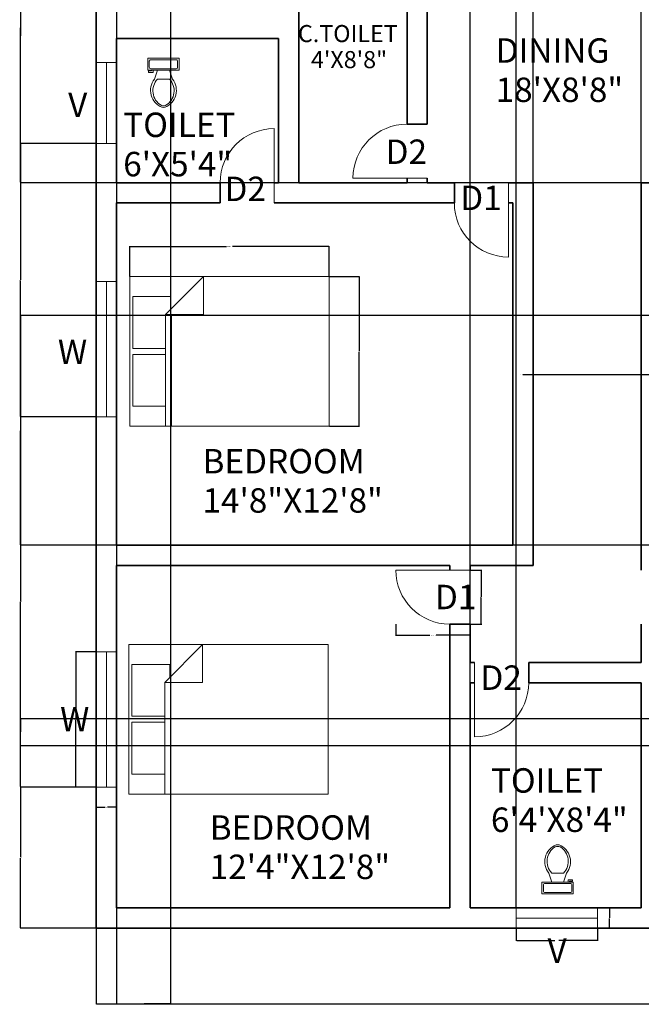
# Model space of a CAD drawing. Units: feet. Extents: x 1681 to 2398, y 1737 to 2411.
# Tile 1 of 4: x 1681 to 1957, y 1737 to 2174. Entities that reach past the tile are written whole.
import ezdxf

# ---------------------------------------------------------------- set-up
doc = ezdxf.new("R2010")
doc.units = ezdxf.units.FT
for name, color, linetype, lineweight in [('A-ANNO-DIMS', 2, 'Continuous', 18), ('A-ANNO-TEXT', 7, 'Continuous', 18), ('A-AREA-IDEN', 7, 'Continuous', 18), ('A-DOOR', 3, 'Continuous', 18), ('A-FLOR-FIXT', 9, 'Continuous', 18), ('A-FURN', 8, 'Continuous', 13), ('A-GLAZ', 4, 'Continuous', 18), ('A-WALL', 7, 'Continuous', 35)]:
    doc.layers.add(name, color=color, linetype=linetype, lineweight=lineweight)
doc.styles.get("Standard").update_dxf_attribs({"font": 'arial.ttf'})
doc.dimstyles.get("Standard").update_dxf_attribs({"dimtxt": 0.18, "dimasz": 0.18, "dimexe": 0.18, "dimexo": 0.0625, "dimgap": 0.09, "dimtad": 0, "dimtih": 1, "dimtoh": 1, "dimdec": 4, "dimzin": 0, "dimdsep": 46, "dimtxsty": 'Standard', "dimcen": 0.09, "dimadec": 0, "dimazin": 0, "dimtfac": 1, "dimtdec": 4, "dimtofl": 0, "dimtmove": 0, "dimatfit": 3, "dimfxl": 1, "dimtolj": 1, "dimtzin": 0, "dimarcsym": 0})

# ---------------------------------------------------------------- blocks, each defined once
blk = doc.blocks.new('Toilet - top')
for p, q in [((9.5, -6), (9.5, -2)), ((-10, -8.5), (-8, -8.5)), ((-10, -9.5), (-10, -8.5)), ((-7, -9.5), (-10, -9.5)), ((-8, -8.5), (-8, -8)), ((-7, -8), (-7, -9.5)), ((-4, -8), (-6, -14)), ((4, -8), (6, -14)), ((4, -14), (-4, -14))]:
    blk.add_line(p, q)
blk.add_lwpolyline([(10.5, -8), (10.5, 0), (-10.5, 0), (-10.5, -8)], close=True)
for points in [[(-9.5, -2), (-9.5, -6)], [(8.5, -1), (-8.5, -1)], [(-8.5, -7), (8.5, -7)]]:
    blk.add_lwpolyline(points)
for centre, radius, start, end in [((-8.62, -1.88), 0.884, 81.8699, 188.1301), ((-8.62, -6.12), 0.884, 171.8699, 278.1301), ((8.62, -1.88), 0.884, 351.8699, 98.1301), ((8.62, -6.12), 0.884, 261.8699, 8.1301), ((3.52, -21.58), 12.17, 141.46911, 247.97143), ((4.2, -21.82), 11.33, 136.36773, 238.94682), ((-3.52, -21.58), 12.17, 292.02843, 38.53071), ((-4.2, -21.82), 11.33, 301.05301, 43.63209), ((0, -27.88), 4, 245.73182, 294.26817), ((0, -29), 4, 254.86053, 285.13947)]:
    blk.add_arc(centre, radius, start, end)
blk = doc.blocks.new('Bed - Queen')
for p, q in [((0, -80.00003), (0, 0)), ((0, 0), (59.99999, 0)), ((59.99999, 0), (59.99999, -80.00003)), ((7.99999, -1.2), (28.79998, -1.2)), ((7.99999, -14.4), (7.99999, -1.2)), ((28.79998, -1.2), (28.79998, -14.4)), ((31.19999, -1.2), (51.99999, -1.2)), ((31.19999, -14.4), (31.19999, -1.2)), ((51.99999, -1.2), (51.99999, -16.4)), ((0, -14.4), (44.8, -14.4)), ((59.99999, -29.6), (44.8, -14.4)), ((44.8, -14.4), (44.8, -29.6)), ((44.8, -16.8), (0, -16.8)), ((51.99999, -16.4), (46.79936, -16.4)), ((44.8, -29.6), (59.99999, -29.6)), ((59.99999, -80.00003), (0, -80.00003))]:
    blk.add_line(p, q)
blk = doc.blocks.new('DOOR-SINGLE-SWING')
blk.add_line((33, 0), (0, 0))
blk.add_arc((9, 0), 24, 0, 90)
blk = doc.blocks.new('WINDOW-STANDARD')
for p, q in [((0, 9), (0, 0)), ((60, 9), (60, 0)), ((0, 4.5), (60, 4.5))]:
    blk.add_line(p, q)
blk = doc.blocks.new('WINDOW-VENTILATOR')
for p, q in [((0, 9), (0, 0)), ((36, 9), (36, 0)), ((0, 4.5), (36, 4.5))]:
    blk.add_line(p, q)
blk = doc.blocks.new('*D14')
at = {"layer": 'A-ANNO-DIMS', "color": 0, "lineweight": -2, "transparency": 16777216}
for p, q in [((1847.74, 1905.99), (1847.74, 1900.92)), ((1880.74, 1905.99), (1880.74, 1900.92)), ((1847.92, 1901.1), (1862.8, 1901.1)), ((1880.56, 1901.1), (1865.68, 1901.1))]:
    blk.add_line(p, q, dxfattribs=at)
at = {"layer": 'A-ANNO-DIMS', "color": 0, "transparency": 16777216}
for points in [[(1847.92, 1901.13), (1847.92, 1901.07), (1847.74, 1901.1)], [(1880.56, 1901.13), (1880.56, 1901.07), (1880.74, 1901.1)]]:
    blk.add_solid(points, dxfattribs=at)
at = {"layer": 'Defpoints', "color": 0, "transparency": 16777216}
for p in [(1847.74, 1906.05), (1880.74, 1906.05), (1847.74, 1901.1)]:
    blk.add_point(p, dxfattribs=at)
at = {"layer": 'A-ANNO-DIMS', "color": 0, "transparency": 16777216, "insert": (1864.24, 1901.1), "char_height": 0.18, "attachment_point": 5}
blk.add_mtext('\\A1;SINGLE DOOR 33 TYP.', dxfattribs=at)
blk = doc.blocks.new('*D15')
at = {"layer": 'A-ANNO-DIMS', "color": 0, "lineweight": -2, "transparency": 16777216}
for p, q in [((1880.8, 1930.05), (1885.87, 1930.05)), ((1885.69, 1929.87), (1885.69, 1918.23)), ((1885.69, 1906.23), (1885.69, 1917.87)), ((1880.8, 1906.05), (1885.87, 1906.05))]:
    blk.add_line(p, q, dxfattribs=at)
at = {"layer": 'A-ANNO-DIMS', "color": 0, "transparency": 16777216}
for points in [[(1885.66, 1929.87), (1885.72, 1929.87), (1885.69, 1930.05)], [(1885.66, 1906.23), (1885.72, 1906.23), (1885.69, 1906.05)]]:
    blk.add_solid(points, dxfattribs=at)
at = {"layer": 'Defpoints', "color": 0, "transparency": 16777216}
for p in [(1880.74, 1930.05), (1880.74, 1906.05), (1885.69, 1906.05)]:
    blk.add_point(p, dxfattribs=at)
at = {"layer": 'A-ANNO-DIMS', "color": 0, "transparency": 16777216, "insert": (1885.69, 1918.05), "char_height": 0.18, "attachment_point": 5}
blk.add_mtext('\\A1;24 TYP.', dxfattribs=at)
blk = doc.blocks.new('*D16')
at = {"layer": 'A-ANNO-DIMS', "color": 0, "lineweight": -2, "transparency": 16777216}
for p, q in [((1714.68, 1893.73), (1705.56, 1893.73)), ((1705.74, 1893.55), (1705.74, 1863.91)), ((1705.74, 1833.91), (1705.74, 1863.54)), ((1714.68, 1833.73), (1705.56, 1833.73))]:
    blk.add_line(p, q, dxfattribs=at)
at = {"layer": 'A-ANNO-DIMS', "color": 0, "transparency": 16777216}
for points in [[(1705.71, 1893.55), (1705.77, 1893.55), (1705.74, 1893.73)], [(1705.71, 1833.91), (1705.77, 1833.91), (1705.74, 1833.73)]]:
    blk.add_solid(points, dxfattribs=at)
at = {"layer": 'Defpoints', "color": 0, "transparency": 16777216}
for p in [(1714.74, 1893.73), (1705.74, 1833.73), (1714.74, 1833.73)]:
    blk.add_point(p, dxfattribs=at)
at = {"layer": 'A-ANNO-DIMS', "color": 0, "transparency": 16777216, "insert": (1705.74, 1863.73), "char_height": 0.18, "attachment_point": 5}
blk.add_mtext('\\A1;WINDOW 60 TYP.', dxfattribs=at)
blk = doc.blocks.new('*D17')
at = {"layer": 'A-ANNO-DIMS', "color": 0, "lineweight": -2, "transparency": 16777216}
for p, q in [((1714.74, 1833.67), (1714.74, 1824.55)), ((1723.74, 1833.67), (1723.74, 1824.55)), ((1714.92, 1824.73), (1718.78, 1824.73)), ((1723.56, 1824.73), (1719.7, 1824.73))]:
    blk.add_line(p, q, dxfattribs=at)
at = {"layer": 'A-ANNO-DIMS', "color": 0, "transparency": 16777216}
for points in [[(1714.92, 1824.76), (1714.92, 1824.7), (1714.74, 1824.73)], [(1723.56, 1824.76), (1723.56, 1824.7), (1723.74, 1824.73)]]:
    blk.add_solid(points, dxfattribs=at)
at = {"layer": 'Defpoints', "color": 0, "transparency": 16777216}
for p in [(1714.74, 1833.73), (1723.74, 1833.73), (1723.74, 1824.73)]:
    blk.add_point(p, dxfattribs=at)
at = {"layer": 'A-ANNO-DIMS', "color": 0, "transparency": 16777216, "insert": (1719.24, 1824.73), "char_height": 0.18, "attachment_point": 5}
blk.add_mtext('\\A1;9 TYP.', dxfattribs=at)
blk = doc.blocks.new('*D18')
at = {"layer": 'A-ANNO-DIMS', "color": 0, "lineweight": -2, "transparency": 16777216}
for p, q in [((1729.63, 2060.43), (1729.63, 2073.83)), ((1729.81, 2073.65), (1772.6, 2073.65)), ((1818, 2073.65), (1775.21, 2073.65)), ((1818.18, 2060.43), (1818.18, 2073.83))]:
    blk.add_line(p, q, dxfattribs=at)
at = {"layer": 'A-ANNO-DIMS', "color": 0, "transparency": 16777216}
for points in [[(1729.81, 2073.68), (1729.81, 2073.62), (1729.63, 2073.65)], [(1818, 2073.68), (1818, 2073.62), (1818.18, 2073.65)]]:
    blk.add_solid(points, dxfattribs=at)
at = {"layer": 'Defpoints', "color": 0, "transparency": 16777216}
for p in [(1729.63, 2073.65), (1729.63, 2060.36), (1818.18, 2060.36)]:
    blk.add_point(p, dxfattribs=at)
at = {"layer": 'A-ANNO-DIMS', "color": 0, "transparency": 16777216, "insert": (1773.9, 2073.65), "char_height": 0.18, "attachment_point": 5}
blk.add_mtext('\\A1;QUEEN BED 89 TYP.', dxfattribs=at)
blk = doc.blocks.new('*D19')
at = {"layer": 'A-ANNO-DIMS', "color": 0, "lineweight": -2, "transparency": 16777216}
for p, q in [((1818.24, 2060.36), (1831.64, 2060.36)), ((1831.46, 2060.18), (1831.46, 2027.34)), ((1831.46, 1994.14), (1831.46, 2026.98)), ((1818.24, 1993.96), (1831.64, 1993.96))]:
    blk.add_line(p, q, dxfattribs=at)
at = {"layer": 'A-ANNO-DIMS', "color": 0, "transparency": 16777216}
for points in [[(1831.43, 2060.18), (1831.49, 2060.18), (1831.46, 2060.36)], [(1831.43, 1994.14), (1831.49, 1994.14), (1831.46, 1993.96)]]:
    blk.add_solid(points, dxfattribs=at)
at = {"layer": 'Defpoints', "color": 0, "transparency": 16777216}
for p in [(1818.18, 2060.36), (1831.46, 2060.36), (1818.18, 1993.96)]:
    blk.add_point(p, dxfattribs=at)
at = {"layer": 'A-ANNO-DIMS', "color": 0, "transparency": 16777216, "insert": (1831.46, 2027.16), "char_height": 0.18, "attachment_point": 5}
blk.add_mtext('\\A1;66 TYP.', dxfattribs=at)
blk = doc.blocks.new('*D22')
at = {"layer": 'A-ANNO-DIMS', "color": 0, "lineweight": -2, "transparency": 16777216}
for p, q in [((1901.24, 1770.99), (1901.24, 1765.47)), ((1937.24, 1770.99), (1937.24, 1765.47)), ((1901.42, 1765.65), (1918.34, 1765.65)), ((1937.06, 1765.65), (1920.14, 1765.65))]:
    blk.add_line(p, q, dxfattribs=at)
at = {"layer": 'A-ANNO-DIMS', "color": 0, "transparency": 16777216}
for points in [[(1901.42, 1765.68), (1901.42, 1765.62), (1901.24, 1765.65)], [(1937.06, 1765.68), (1937.06, 1765.62), (1937.24, 1765.65)]]:
    blk.add_solid(points, dxfattribs=at)
at = {"layer": 'Defpoints', "color": 0, "transparency": 16777216}
for p in [(1901.24, 1771.05), (1937.24, 1771.05), (1937.24, 1765.65)]:
    blk.add_point(p, dxfattribs=at)
at = {"layer": 'A-ANNO-DIMS', "color": 0, "transparency": 16777216, "insert": (1919.24, 1765.65), "char_height": 0.18, "attachment_point": 5}
blk.add_mtext('\\A1;VENT 36 TYP.', dxfattribs=at)
blk = doc.blocks.new('*D23')
at = {"layer": 'A-ANNO-DIMS', "color": 0, "lineweight": -2, "transparency": 16777216}
for p, q in [((1937.3, 1780.05), (1942.82, 1780.05)), ((1942.64, 1779.87), (1942.64, 1775.73)), ((1942.64, 1771.23), (1942.64, 1775.37)), ((1937.3, 1771.05), (1942.82, 1771.05))]:
    blk.add_line(p, q, dxfattribs=at)
at = {"layer": 'A-ANNO-DIMS', "color": 0, "transparency": 16777216}
for points in [[(1942.61, 1779.87), (1942.67, 1779.87), (1942.64, 1780.05)], [(1942.61, 1771.23), (1942.67, 1771.23), (1942.64, 1771.05)]]:
    blk.add_solid(points, dxfattribs=at)
at = {"layer": 'Defpoints', "color": 0, "transparency": 16777216}
for p in [(1937.24, 1780.05), (1942.64, 1780.05), (1937.24, 1771.05)]:
    blk.add_point(p, dxfattribs=at)
at = {"layer": 'A-ANNO-DIMS', "color": 0, "transparency": 16777216, "insert": (1942.64, 1775.55), "char_height": 0.18, "attachment_point": 5}
blk.add_mtext('\\A1;9 TYP.', dxfattribs=at)
blk = doc.blocks.new('*D40')
at = {"layer": 'A-ANNO-DIMS', "color": 0, "lineweight": -2, "transparency": 16777216}
for p, q in [((1714.74, 1770.99), (1714.74, 1737.27)), ((2339.74, 1770.99), (2339.74, 1737.27)), ((1714.92, 1737.45), (2026.95, 1737.45)), ((2339.56, 1737.45), (2027.53, 1737.45))]:
    blk.add_line(p, q, dxfattribs=at)
at = {"layer": 'A-ANNO-DIMS', "color": 0, "transparency": 16777216}
for points in [[(1714.92, 1737.48), (1714.92, 1737.42), (1714.74, 1737.45)], [(2339.56, 1737.48), (2339.56, 1737.42), (2339.74, 1737.45)]]:
    blk.add_solid(points, dxfattribs=at)
at = {"layer": 'Defpoints', "color": 0, "transparency": 16777216}
for p in [(1714.74, 1771.05), (2339.74, 1771.05), (2339.74, 1737.45)]:
    blk.add_point(p, dxfattribs=at)
at = {"layer": 'A-ANNO-DIMS', "color": 0, "transparency": 16777216, "insert": (2027.24, 1737.45), "char_height": 0.18, "attachment_point": 5}
blk.add_mtext('\\A1;625', dxfattribs=at)
blk = doc.blocks.new('*D46')
at = {"layer": 'A-ANNO-DIMS', "color": 0, "lineweight": -2, "transparency": 16777216}
for p, q in [((1714.68, 1833.73), (1680.96, 1833.73)), ((1681.14, 1833.55), (1681.14, 1802.57)), ((1681.14, 1771.23), (1681.14, 1802.21)), ((1714.68, 1771.05), (1680.96, 1771.05))]:
    blk.add_line(p, q, dxfattribs=at)
at = {"layer": 'A-ANNO-DIMS', "color": 0, "transparency": 16777216}
for points in [[(1681.11, 1833.55), (1681.17, 1833.55), (1681.14, 1833.73)], [(1681.11, 1771.23), (1681.17, 1771.23), (1681.14, 1771.05)]]:
    blk.add_solid(points, dxfattribs=at)
at = {"layer": 'Defpoints', "color": 0, "transparency": 16777216}
for p in [(1681.14, 1833.73), (1714.74, 1833.73), (1714.74, 1771.05)]:
    blk.add_point(p, dxfattribs=at)
at = {"layer": 'A-ANNO-DIMS', "color": 0, "transparency": 16777216, "insert": (1681.14, 1802.39), "char_height": 0.18, "attachment_point": 5}
blk.add_mtext('\\A1;62.68', dxfattribs=at)
blk = doc.blocks.new('*D47')
at = {"layer": 'A-ANNO-DIMS', "color": 0, "lineweight": -2, "transparency": 16777216}
for p, q in [((1714.68, 1998.11), (1680.96, 1998.11)), ((1681.14, 1997.93), (1681.14, 1916.1)), ((1681.14, 1833.91), (1681.14, 1915.74)), ((1714.68, 1833.73), (1680.96, 1833.73))]:
    blk.add_line(p, q, dxfattribs=at)
at = {"layer": 'A-ANNO-DIMS', "color": 0, "transparency": 16777216}
for points in [[(1681.11, 1997.93), (1681.17, 1997.93), (1681.14, 1998.11)], [(1681.11, 1833.91), (1681.17, 1833.91), (1681.14, 1833.73)]]:
    blk.add_solid(points, dxfattribs=at)
at = {"layer": 'Defpoints', "color": 0, "transparency": 16777216}
for p in [(1681.14, 1998.11), (1714.74, 1998.11), (1714.74, 1833.73)]:
    blk.add_point(p, dxfattribs=at)
at = {"layer": 'A-ANNO-DIMS', "color": 0, "transparency": 16777216, "insert": (1681.14, 1915.92), "char_height": 0.18, "attachment_point": 5}
blk.add_mtext('\\A1;164.38', dxfattribs=at)
blk = doc.blocks.new('*D48')
at = {"layer": 'A-ANNO-DIMS', "color": 0, "lineweight": -2, "transparency": 16777216}
for p, q in [((1714.68, 2119.4), (1680.96, 2119.4)), ((1681.14, 2119.22), (1681.14, 2058.93)), ((1681.14, 1998.29), (1681.14, 2058.57)), ((1714.68, 1998.11), (1680.96, 1998.11))]:
    blk.add_line(p, q, dxfattribs=at)
at = {"layer": 'A-ANNO-DIMS', "color": 0, "transparency": 16777216}
for points in [[(1681.11, 2119.22), (1681.17, 2119.22), (1681.14, 2119.4)], [(1681.11, 1998.29), (1681.17, 1998.29), (1681.14, 1998.11)]]:
    blk.add_solid(points, dxfattribs=at)
at = {"layer": 'Defpoints', "color": 0, "transparency": 16777216}
for p in [(1681.14, 2119.4), (1714.74, 2119.4), (1714.74, 1998.11)]:
    blk.add_point(p, dxfattribs=at)
at = {"layer": 'A-ANNO-DIMS', "color": 0, "transparency": 16777216, "insert": (1681.14, 2058.75), "char_height": 0.18, "attachment_point": 5}
blk.add_mtext('\\A1;121.29', dxfattribs=at)
blk = doc.blocks.new('*D49')
at = {"layer": 'A-ANNO-DIMS', "color": 0, "lineweight": -2, "transparency": 16777216}
for p, q in [((1714.68, 2222.05), (1680.96, 2222.05)), ((1681.14, 2221.87), (1681.14, 2170.9)), ((1681.14, 2119.58), (1681.14, 2170.54)), ((1714.68, 2119.4), (1680.96, 2119.4))]:
    blk.add_line(p, q, dxfattribs=at)
at = {"layer": 'A-ANNO-DIMS', "color": 0, "transparency": 16777216}
for points in [[(1681.11, 2221.87), (1681.17, 2221.87), (1681.14, 2222.05)], [(1681.11, 2119.58), (1681.17, 2119.58), (1681.14, 2119.4)]]:
    blk.add_solid(points, dxfattribs=at)
at = {"layer": 'Defpoints', "color": 0, "transparency": 16777216}
for p in [(1681.14, 2222.05), (1714.74, 2222.05), (1714.74, 2119.4)]:
    blk.add_point(p, dxfattribs=at)
at = {"layer": 'A-ANNO-DIMS', "color": 0, "transparency": 16777216, "insert": (1681.14, 2170.72), "char_height": 0.18, "attachment_point": 5}
blk.add_mtext('\\A1;102.65', dxfattribs=at)
blk = doc.blocks.new('*D50')
at = {"layer": 'A-ANNO-DIMS', "color": 0, "lineweight": -2, "transparency": 16777216}
for p, q in [((2330.68, 2232.39), (1680.96, 2232.39)), ((1681.14, 2232.21), (1681.14, 2167.4)), ((1681.14, 2102.23), (1681.14, 2167.04)), ((2330.68, 2102.05), (1680.96, 2102.05))]:
    blk.add_line(p, q, dxfattribs=at)
at = {"layer": 'A-ANNO-DIMS', "color": 0, "transparency": 16777216}
for points in [[(1681.11, 2232.21), (1681.17, 2232.21), (1681.14, 2232.39)], [(1681.11, 2102.23), (1681.17, 2102.23), (1681.14, 2102.05)]]:
    blk.add_solid(points, dxfattribs=at)
at = {"layer": 'Defpoints', "color": 0, "transparency": 16777216}
for p in [(1681.14, 2232.39), (2330.74, 2232.39), (2330.74, 2102.05)]:
    blk.add_point(p, dxfattribs=at)
at = {"layer": 'A-ANNO-DIMS', "color": 0, "transparency": 16777216, "insert": (1681.14, 2167.22), "char_height": 0.18, "attachment_point": 5}
blk.add_mtext('\\A1;130.34', dxfattribs=at)
blk = doc.blocks.new('*D51')
at = {"layer": 'A-ANNO-DIMS', "color": 0, "lineweight": -2, "transparency": 16777216}
for p, q in [((1880.74, 1780.11), (1880.74, 2410.83)), ((1880.92, 2410.65), (1890.66, 2410.65)), ((1901.06, 2410.65), (1891.32, 2410.65)), ((1901.24, 1780.11), (1901.24, 2410.83))]:
    blk.add_line(p, q, dxfattribs=at)
at = {"layer": 'A-ANNO-DIMS', "color": 0, "transparency": 16777216}
for points in [[(1880.92, 2410.68), (1880.92, 2410.62), (1880.74, 2410.65)], [(1901.06, 2410.68), (1901.06, 2410.62), (1901.24, 2410.65)]]:
    blk.add_solid(points, dxfattribs=at)
at = {"layer": 'Defpoints', "color": 0, "transparency": 16777216}
for p in [(1901.24, 2410.65), (1880.74, 1780.05), (1901.24, 1780.05)]:
    blk.add_point(p, dxfattribs=at)
at = {"layer": 'A-ANNO-DIMS', "color": 0, "transparency": 16777216, "insert": (1890.99, 2410.65), "char_height": 0.18, "attachment_point": 5}
blk.add_mtext('\\A1;20.5', dxfattribs=at)
blk = doc.blocks.new('*D57')
at = {"layer": 'A-ANNO-DIMS', "color": 0, "lineweight": -2, "transparency": 16777216}
for p, q in [((2153.68, 2043.05), (1680.96, 2043.05)), ((1681.14, 2042.87), (1681.14, 1992.23)), ((1681.14, 1941.23), (1681.14, 1991.87)), ((2153.68, 1941.05), (1680.96, 1941.05))]:
    blk.add_line(p, q, dxfattribs=at)
at = {"layer": 'A-ANNO-DIMS', "color": 0, "transparency": 16777216}
for points in [[(1681.11, 2042.87), (1681.17, 2042.87), (1681.14, 2043.05)], [(1681.11, 1941.23), (1681.17, 1941.23), (1681.14, 1941.05)]]:
    blk.add_solid(points, dxfattribs=at)
at = {"layer": 'Defpoints', "color": 0, "transparency": 16777216}
for p in [(1681.14, 2043.05), (2153.74, 2043.05), (2153.74, 1941.05)]:
    blk.add_point(p, dxfattribs=at)
at = {"layer": 'A-ANNO-DIMS', "color": 0, "transparency": 16777216, "insert": (1681.14, 1992.05), "char_height": 0.18, "attachment_point": 5}
blk.add_mtext('\\A1;102', dxfattribs=at)
blk = doc.blocks.new('*D58')
at = {"layer": 'A-ANNO-DIMS', "color": 0, "lineweight": -2, "transparency": 16777216}
for p, q in [((1908.74, 1932.11), (1908.74, 2410.83)), ((1908.92, 2410.65), (1932.52, 2410.65)), ((1956.56, 2410.65), (1932.96, 2410.65)), ((1956.74, 1932.11), (1956.74, 2410.83))]:
    blk.add_line(p, q, dxfattribs=at)
at = {"layer": 'A-ANNO-DIMS', "color": 0, "transparency": 16777216}
for points in [[(1908.92, 2410.68), (1908.92, 2410.62), (1908.74, 2410.65)], [(1956.56, 2410.68), (1956.56, 2410.62), (1956.74, 2410.65)]]:
    blk.add_solid(points, dxfattribs=at)
at = {"layer": 'Defpoints', "color": 0, "transparency": 16777216}
for p in [(1956.74, 2410.65), (1908.74, 1932.05), (1956.74, 1932.05)]:
    blk.add_point(p, dxfattribs=at)
at = {"layer": 'A-ANNO-DIMS', "color": 0, "transparency": 16777216, "insert": (1932.74, 2410.65), "char_height": 0.18, "attachment_point": 5}
blk.add_mtext('\\A1;48', dxfattribs=at)
blk = doc.blocks.new('*D60')
at = {"layer": 'A-ANNO-DIMS', "color": 0, "lineweight": -2, "transparency": 16777216}
for p, q in [((1723.74, 2245.99), (1723.74, 1737.27)), ((1747.74, 2245.99), (1747.74, 1737.27)), ((1723.92, 1737.45), (1735.52, 1737.45)), ((1747.56, 1737.45), (1735.96, 1737.45))]:
    blk.add_line(p, q, dxfattribs=at)
at = {"layer": 'A-ANNO-DIMS', "color": 0, "transparency": 16777216}
for points in [[(1723.92, 1737.48), (1723.92, 1737.42), (1723.74, 1737.45)], [(1747.56, 1737.48), (1747.56, 1737.42), (1747.74, 1737.45)]]:
    blk.add_solid(points, dxfattribs=at)
at = {"layer": 'Defpoints', "color": 0, "transparency": 16777216}
for p in [(1723.74, 2246.05), (1747.74, 2246.05), (1747.74, 1737.45)]:
    blk.add_point(p, dxfattribs=at)
at = {"layer": 'A-ANNO-DIMS', "color": 0, "transparency": 16777216, "insert": (1735.74, 1737.45), "char_height": 0.18, "attachment_point": 5}
blk.add_mtext('\\A1;24', dxfattribs=at)
blk = doc.blocks.new('*D62')
at = {"layer": 'A-ANNO-DIMS', "color": 0, "lineweight": -2, "transparency": 16777216}
for p, q in [((2098.68, 1864.05), (1680.96, 1864.05)), ((1681.14, 1863.87), (1681.14, 1858.23)), ((1681.14, 1852.23), (1681.14, 1857.87)), ((2098.68, 1852.05), (1680.96, 1852.05))]:
    blk.add_line(p, q, dxfattribs=at)
at = {"layer": 'A-ANNO-DIMS', "color": 0, "transparency": 16777216}
for points in [[(1681.11, 1863.87), (1681.17, 1863.87), (1681.14, 1864.05)], [(1681.11, 1852.23), (1681.17, 1852.23), (1681.14, 1852.05)]]:
    blk.add_solid(points, dxfattribs=at)
at = {"layer": 'Defpoints', "color": 0, "transparency": 16777216}
for p in [(1681.14, 1864.05), (2098.74, 1864.05), (2098.74, 1852.05)]:
    blk.add_point(p, dxfattribs=at)
at = {"layer": 'A-ANNO-DIMS', "color": 0, "transparency": 16777216, "insert": (1681.14, 1858.05), "char_height": 0.18, "attachment_point": 5}
blk.add_mtext('\\A1;12', dxfattribs=at)
blk = doc.blocks.new('*D65')
at = {"layer": 'A-ANNO-DIMS', "color": 0, "lineweight": -2, "transparency": 16777216}
for p, q in [((1904.14, 2016.92), (1977.25, 2016.92)), ((2099.48, 2016.93), (2099.66, 2016.93)), ((2099.57, 2016.84), (2099.57, 2017.02))]:
    blk.add_line(p, q, dxfattribs=at)
at = {"layer": 'A-ANNO-DIMS', "color": 0, "transparency": 16777216}
blk.add_solid([(1977.25, 2016.95), (1977.25, 2016.89), (1977.43, 2016.92)], dxfattribs=at)
at = {"layer": 'Defpoints', "color": 0, "transparency": 16777216}
for p in [(1977.43, 2016.92), (2099.57, 2016.93)]:
    blk.add_point(p, dxfattribs=at)
at = {"layer": 'A-ANNO-DIMS', "color": 0, "transparency": 16777216, "insert": (1903.4, 2016.92), "char_height": 0.18, "attachment_point": 5}
blk.add_mtext('\\A1;2X R122.14', dxfattribs=at)

msp = doc.modelspace()

# ---------------------------------------------------------------- linework, layer by layer
at = {"layer": 'A-WALL'}
for p, q in [((1714.7402, 2222.0485), (1714.7402, 2102.0485)), ((1714.7402, 2222.0485), (1714.7402, 1771.0485)), ((1861.7402, 2220.0485), (1861.7402, 2128.0485)), ((1804.7402, 2102.0485), (1804.7402, 2211.0485)), ((1852.7402, 2211.0485), (1852.7402, 2128.0485)), ((1723.7402, 2166.0485), (1795.7402, 2166.0485)), ((1723.7402, 2166.0485), (1723.7402, 2102.0485)), ((1795.7402, 2102.0485), (1795.7402, 2166.0485)), ((1852.7402, 2128.0485), (1861.7402, 2128.0485)), ((1852.7402, 2104.0485), (1852.7402, 2102.0485)), ((1861.7402, 2104.0485), (1861.7402, 2102.0485)), ((1723.7402, 2102.0485), (1769.7402, 2102.0485)), ((1769.7402, 2093.0485), (1769.7402, 2102.0485)), ((1793.7402, 2102.0485), (1795.7402, 2102.0485)), ((1804.7402, 2102.0485), (1852.7402, 2102.0485)), ((1861.7402, 2102.0485), (1873.7402, 2102.0485)), ((1873.7402, 2093.0485), (1873.7402, 2102.0485)), ((1897.7402, 2102.0485), (1908.7402, 2102.0485)), ((1908.7402, 1932.0485), (1908.7402, 2102.0485)), ((1956.7402, 2089.0485), (1956.7402, 2102.0485)), ((1956.7402, 2102.0485), (2042.3686, 2102.0485)), ((1723.7402, 2093.0485), (1769.7402, 2093.0485)), ((1723.7402, 2093.0485), (1723.7402, 1941.0485)), ((1793.7402, 2093.0485), (1873.7402, 2093.0485)), ((1804.7402, 2093.0485), (1852.7402, 2093.0485)), ((1897.7402, 2093.0485), (1899.7402, 2093.0485)), ((1899.7402, 1941.0485), (1899.7402, 2093.0485)), ((1956.7402, 1941.0485), (1956.7402, 2089.0485)), ((1723.7402, 1941.0485), (1899.7402, 1941.0485)), ((1956.7402, 1932.0485), (1956.7402, 1941.0485)), ((1714.7402, 1932.0485), (1714.7402, 1771.0485)), ((1723.7402, 1932.0485), (1871.7402, 1932.0485)), ((1723.7402, 1932.0485), (1723.7402, 1780.0485)), ((1871.7402, 1930.0485), (1871.7402, 1932.0485)), ((1880.7402, 1932.0485), (1908.7402, 1932.0485)), ((1880.7402, 1930.0485), (1880.7402, 1932.0485)), ((1956.7402, 1932.0485), (1956.7402, 1930.0485)), ((1871.7402, 1780.0485), (1871.7402, 1906.0485)), ((1871.7402, 1906.0485), (1880.7402, 1906.0485)), ((1880.7402, 1889.0485), (1880.7402, 1906.0485)), ((1956.7402, 1906.0485), (1956.7402, 1889.0485)), ((1882.7402, 1889.0485), (1880.7402, 1889.0485)), ((1956.7402, 1889.0485), (1906.7402, 1889.0485)), ((1906.7402, 1880.0485), (1906.7402, 1889.0485)), ((1880.7402, 1780.0485), (1880.7402, 1880.0485)), ((1882.7402, 1880.0485), (1880.7402, 1880.0485)), ((1956.7402, 1880.0485), (1906.7402, 1880.0485)), ((1956.7402, 1780.0485), (1956.7402, 1880.0485)), ((1956.7402, 1880.0485), (1956.7402, 1877.7891)), ((1723.7402, 1780.0485), (1871.7402, 1780.0485)), ((1880.7402, 1780.0485), (1956.7402, 1780.0485)), ((1714.7402, 1771.0485), (2194.7402, 1771.0485)), ((1880.7402, 1771.0485), (2194.7402, 1771.0485))]:
    msp.add_line(p, q, dxfattribs=at)

# ---------------------------------------------------------------- block references
at = {"layer": 'A-DOOR'}
for p, rotation in [((1793.7402, 2093.0485), 89.99999999999955), ((1880.7402, 1930.0485), 180), ((1882.7402, 1889.0485), 269.9999999999992)]:
    msp.add_blockref('DOOR-SINGLE-SWING', p, dxfattribs=dict(at, rotation=rotation))
at = {"layer": 'A-DOOR', "extrusion": (0, 0, -1), "zscale": -1}
msp.add_blockref('DOOR-SINGLE-SWING', (-1861.7402, 2104.0485), dxfattribs=at)
at = {"layer": 'A-DOOR', "extrusion": (0, 0, -1), "zscale": -1, "rotation": 269.9999999999986}
msp.add_blockref('DOOR-SINGLE-SWING', (-1897.7402, 2102.0485), dxfattribs=at)
at = {"layer": 'A-FLOR-FIXT', "xscale": 0.6624009790136799, "yscale": 0.6624009790136799, "zscale": 0.6624009790136799}
msp.add_blockref('Toilet - top', (1744.6057, 2157.2837), dxfattribs=at)
at = {"layer": 'A-FLOR-FIXT', "xscale": 0.6624009790136799, "yscale": 0.6624009790136799, "zscale": 0.6624009790136799, "rotation": 180}
msp.add_blockref('Toilet - top', (1919.598, 1786.2711), dxfattribs=at)
at = {"layer": 'A-FURN', "xscale": 1.106801235632363, "yscale": 1.106801235632363, "zscale": 1.106801235632363, "rotation": 89.99999999999999}
for p in [(1729.6323, 1993.9554), (1729.2265, 1830.6232)]:
    msp.add_blockref('Bed - Queen', p, dxfattribs=at)
at = {"layer": 'A-GLAZ'}
for name, p, rotation in [('WINDOW-VENTILATOR', (1714.7402, 2155.3956), 270.0000000000041), ('WINDOW-STANDARD', (1714.7402, 2058.1093), 270.0000000000009), ('WINDOW-STANDARD', (1714.7402, 1893.7275), 270.0000000000008)]:
    msp.add_blockref(name, p, dxfattribs=dict(at, rotation=rotation))
msp.add_blockref('WINDOW-VENTILATOR', (1901.2406, 1771.0485), dxfattribs=at)

# ---------------------------------------------------------------- texts
at = {"layer": 'A-ANNO-TEXT'}
for s, height, p in [('V', 10.8568, (1702.2656, 2131.1968)), ('D2', 10.85679, (1843.2087, 2110.3634)), ('D2', 10.85679, (1771.6867, 2093.8777)), ('D1', 10.85679, (1876.3492, 2089.8927)), ('W', 10.8568, (1697.7184, 2021.4917)), ('D1', 10.85679, (1865.1147, 1912.6719)), ('D2', 10.85679, (1885.291, 1876.8683)), ('W', 10.8568, (1698.695, 1858.4701)), ('V', 10.8568, (1915.0925, 1755.6747))]:
    msp.add_text(s, height=height, dxfattribs=at).set_placement(p)
at = {"layer": 'A-AREA-IDEN'}
for s, height, p in [('C.TOILET', 7.58907, (1804.2824, 2164.4602)), ('DINING', 10.85679, (1892.0744, 2155.2995)), ('4\'X8\'8"', 7.58907, (1810.0678, 2152.9004)), ('18\'X8\'8"', 10.85679, (1892.0744, 2137.859)), ('TOILET', 10.85679, (1726.7254, 2122.3135)), ('6\'X5\'4"', 10.85679, (1726.7254, 2104.873)), ('BEDROOM', 10.85679, (1761.9261, 1972.9738)), ('14\'8"X12\'8"', 10.856786, (1761.9261, 1955.5333)), ('TOILET', 10.85679, (1889.9657, 1831.2213)), ('6\'4\'X8\'4"', 10.85679, (1889.9657, 1813.7808)), ('BEDROOM', 10.85679, (1765.1389, 1810.3167)), ('12\'4"X12\'8"', 10.856786, (1765.1389, 1792.8762))]:
    msp.add_text(s, height=height, dxfattribs=at).set_placement(p)

# ---------------------------------------------------------------- dimensions: what is measured, and where the dimension line sits
at = {"layer": 'A-ANNO-DIMS'}
for base, p1, p2, override, picture, middle in [((1901.2406, 2410.6485), (1880.7402, 1780.0485), (1901.2406, 1780.0485), {"dimdec": 1, "dimlfac": 1, "dimrnd": 0, "dimzin": 0, "dimdsep": 46, "dimlunit": 2}, '*D51', (1890.9904, 2410.6485)), ((1956.7402, 2410.6485), (1908.7402, 1932.0485), (1956.7402, 1932.0485), {"dimdec": 0, "dimlfac": 1, "dimrnd": 0, "dimzin": 0, "dimdsep": 46, "dimlunit": 2}, '*D58', (1932.7402, 2410.6485)), ((1747.7402, 1737.4485), (1723.7402, 2246.0485), (1747.7402, 2246.0485), {"dimdec": 0, "dimlfac": 1, "dimrnd": 0, "dimzin": 0, "dimdsep": 46, "dimlunit": 2}, '*D60', (1735.7402, 1737.4485)), ((2339.7402, 1737.4485), (1714.7402, 1771.0485), (2339.7402, 1771.0485), {"dimdec": 0, "dimlfac": 1, "dimrnd": 0, "dimzin": 0, "dimdsep": 46, "dimlunit": 2}, '*D40', (2027.2402, 1737.4485))]:
    dim = msp.add_linear_dim(base=base, p1=p1, p2=p2, dimstyle='Standard', override=override, dxfattribs=at)
    dim.commit()
    dim.dimension.update_dxf_attribs({"geometry": picture, "text_midpoint": middle})
for base, p1, p2, override, picture, middle in [((1681.1402, 2232.3872), (2330.7402, 2102.0485), (2330.7402, 2232.3872), {"dimdec": 2, "dimlfac": 1, "dimrnd": 0, "dimzin": 0, "dimdsep": 46, "dimlunit": 2}, '*D50', (1681.1402, 2167.2178)), ((1681.1402, 2222.0485), (1714.7402, 2119.3956), (1714.7402, 2222.0485), {"dimdec": 2, "dimlfac": 1, "dimrnd": 0, "dimzin": 0, "dimdsep": 46, "dimlunit": 2}, '*D49', (1681.1402, 2170.722)), ((1681.1402, 2119.3956), (1714.7402, 1998.1093), (1714.7402, 2119.3956), {"dimdec": 2, "dimlfac": 1, "dimrnd": 0, "dimzin": 0, "dimdsep": 46, "dimlunit": 2}, '*D48', (1681.1402, 2058.7524)), ((1681.1402, 2043.0485), (2153.7402, 1941.0485), (2153.7402, 2043.0485), {"dimdec": 0, "dimlfac": 1, "dimrnd": 0, "dimzin": 0, "dimdsep": 46, "dimlunit": 2}, '*D57', (1681.1402, 1992.0485)), ((1681.1402, 1998.1093), (1714.7402, 1833.7275), (1714.7402, 1998.1093), {"dimdec": 2, "dimlfac": 1, "dimrnd": 0, "dimzin": 0, "dimdsep": 46, "dimlunit": 2}, '*D47', (1681.1402, 1915.9184)), ((1681.1402, 1864.0485), (2098.7402, 1852.0485), (2098.7402, 1864.0485), {"dimdec": 0, "dimlfac": 1, "dimrnd": 0, "dimzin": 0, "dimdsep": 46, "dimlunit": 2}, '*D62', (1681.1402, 1858.0485)), ((1681.1402, 1833.7275), (1714.7402, 1771.0485), (1714.7402, 1833.7275), {"dimdec": 2, "dimlfac": 1, "dimrnd": 0, "dimzin": 0, "dimdsep": 46, "dimlunit": 2}, '*D46', (1681.1402, 1802.388))]:
    dim = msp.add_linear_dim(base=base, p1=p1, p2=p2, angle=90, dimstyle='Standard', override=override, dxfattribs=at)
    dim.commit()
    dim.dimension.update_dxf_attribs({"geometry": picture, "text_midpoint": middle})
for base, p1, p2, angle, text, picture, middle in [((1729.6323, 2073.6451), (1818.1765, 2060.3635), (1729.6323, 2060.3635), 180, 'QUEEN BED <> TYP.', '*D18', (1773.9044, 2073.6451)), ((1831.4581, 2060.3635), (1818.1765, 1993.9554), (1818.1765, 2060.3635), 90, '<> TYP.', '*D19', (1831.4581, 2027.1594)), ((1885.6902, 1906.0485), (1880.7402, 1930.0485), (1880.7402, 1906.0485), 270, '<> TYP.', '*D15', (1885.6902, 1918.0485)), ((1847.7402, 1901.0985), (1880.7402, 1906.0485), (1847.7402, 1906.0485), 180, 'SINGLE DOOR <> TYP.', '*D14', (1864.2402, 1901.0985)), ((1705.7402, 1833.7275), (1714.7402, 1893.7275), (1714.7402, 1833.7275), 270, 'WINDOW <> TYP.', '*D16', (1705.7402, 1863.7275)), ((1723.7402, 1824.7275), (1714.7402, 1833.7275), (1723.7402, 1833.7275), 0, '<> TYP.', '*D17', (1719.2402, 1824.7275)), ((1942.6406, 1780.0485), (1937.2406, 1771.0485), (1937.2406, 1780.0485), 90, '<> TYP.', '*D23', (1942.6406, 1775.5485))]:
    dim = msp.add_linear_dim(base=base, p1=p1, p2=p2, angle=angle, text=text, dimstyle='Standard', override={"dimdec": 0, "dimlfac": 1, "dimrnd": 0, "dimzin": 0, "dimdsep": 46, "dimlunit": 2}, dxfattribs=at)
    dim.commit()
    dim.dimension.update_dxf_attribs({"geometry": picture, "text_midpoint": middle})
dim = msp.add_radius_dim(center=(2099.5728, 2016.9252), mpoint=(1977.4304, 2016.925), text='2X <>', dimstyle='Standard', override={"dimdec": 2, "dimlfac": 1, "dimrnd": 0, "dimzin": 0, "dimdsep": 46, "dimlunit": 2}, dxfattribs=at)
dim.commit()
dim.dimension.update_dxf_attribs({"geometry": '*D65', "text_midpoint": (1904.145, 2016.9249), "dimtype": 164})
dim = msp.add_linear_dim(base=(1937.2406, 1765.6485), p1=(1901.2406, 1771.0485), p2=(1937.2406, 1771.0485), text='VENT <> TYP.', dimstyle='Standard', override={"dimdec": 0, "dimlfac": 1, "dimrnd": 0, "dimzin": 0, "dimdsep": 46, "dimlunit": 2}, dxfattribs=at)
dim.commit()
dim.dimension.update_dxf_attribs({"geometry": '*D22', "text_midpoint": (1919.2406, 1765.6485)})

doc.saveas('drawing.dxf')
